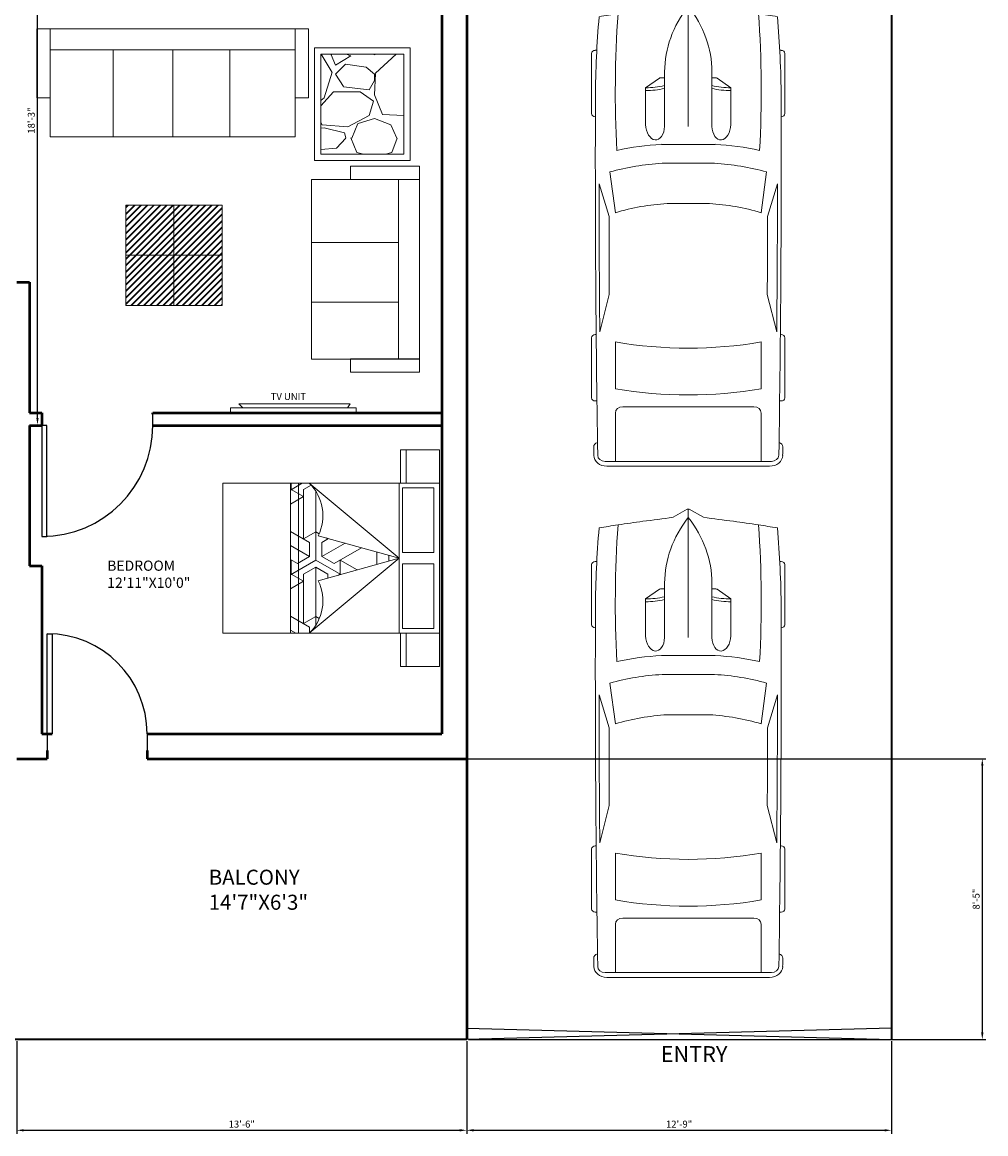
# Model space of a CAD drawing. Units: inches. Extents: x 1455 to 2044, y 1728 to 2439.
# Tile 2 of 4: x 1697 to 2044, y 1728 to 2128. Entities that reach past the tile are written whole.
import ezdxf

# ---------------------------------------------------------------- set-up
doc = ezdxf.new("R2010")
doc.units = ezdxf.units.IN
for name, color, linetype, lineweight in [('A-ANNO-DIMS', 2, 'Continuous', 18), ('A-ANNO-TEXT', 7, 'Continuous', 18), ('A-AREA-IDEN', 7, 'Continuous', 25), ('A-DOOR', 4, 'Continuous', 25), ('A-FURN', 8, 'Continuous', 18), ('A-FURN-PATT', 9, 'Continuous', 13), ('A-WALL', 7, 'Continuous', 50), ('C-PRKG-VEHI', 8, 'Continuous', 13), ('C-PROP', 7, 'Continuous', 35), ('C-SITE-GATE', 1, 'Continuous', 25)]:
    doc.layers.add(name, color=color, linetype=linetype, lineweight=lineweight)
doc.styles.get("Standard").update_dxf_attribs({"font": 'arial.ttf'})
doc.dimstyles.new('ISO-25', dxfattribs={"dimtxt": 2.5, "dimasz": 2.5, "dimexe": 1.25, "dimexo": 0.625, "dimtad": 1, "dimlunit": 3, "dimtxsty": 'Standard', "dimcen": 2.5, "dimadec": 0, "dimazin": 0, "dimtfac": 1, "dimtmove": 0, "dimatfit": 3, "dimfxl": 1, "dimarcsym": 0})

# ---------------------------------------------------------------- blocks, each defined once
blk = doc.blocks.new('*U14')
for p, q in [((0, 0), (0, -6)), ((36, 0), (36, -6))]:
    blk.add_line(p, q)
blk.add_lwpolyline([(0, 0), (0, 36), (1.75, 36), (1.75, 0)], close=True)
blk.add_arc((0, 0), 36, 0, 90)
blk = doc.blocks.new('*U13')
for p, q in [((0, 0), (0, 4)), ((40, 0), (40, 4))]:
    blk.add_line(p, q)
blk.add_lwpolyline([(0, 0), (0, -40), (1.75, -40), (1.75, 0)], close=True)
blk.add_arc((0, 0), 40, 270, 0)
blk = doc.blocks.new('*U19')
for p, q in [((21.1, 37.41), (21.1, 36.83)), ((46.55, 38.89), (22.35, 38.89)), ((47.8, 37.39), (47.8, 37.41)), ((87.99, 31.87), (74.76, 35.92)), ((135.45, 37.07), (135.45, 37.41)), ((136.7, 38.89), (160.9, 38.89)), ((162.15, 37.41), (162.15, 36.77)), ((70.03, 31.54), (86.41, 29.35)), ((134.31, 35.6), (119.29, 31.78)), ((186.47, -33.5), (186.47, 33.5)), ((188.4, -32.76), (188.4, 32.76)), ((138.42, 29.35), (157.25, 29.35)), ((186.47, 29.35), (167.01, 29.35)), ((164.52, 26.39), (164.52, -26.39)), ((32.27, 11.63), (36.13, 17.17)), ((36.13, 17.17), (50.94, 17.17)), ((29.77, 9.51), (51.68, 9.51)), ((32.12, 9.51), (32.12, 11.15)), ((58.92, -10.77), (58.92, 10.77)), ((66.55, -10.53), (66.55, 10.53)), ((186.47, -10.53), (186.47, 10.53)), ((3.27, 6.13), (0.1, 0.41)), ((82.74, 8.5), (82.74, -8.5)), ((0, 0), (51.68, 0)), ((0.1, -0.41), (3.27, -6.13)), ((29.77, -9.51), (51.68, -9.51)), ((32.12, -9.51), (32.12, -11.15)), ((32.27, -11.63), (36.13, -17.17)), ((36.13, -17.17), (50.94, -17.17)), ((86.41, -29.35), (70.03, -31.54)), ((157.25, -29.35), (138.42, -29.35)), ((167.01, -29.35), (186.47, -29.35)), ((87.99, -31.87), (74.76, -35.92)), ((134.31, -35.6), (119.29, -31.78)), ((21.1, -37.41), (21.1, -36.83)), ((46.55, -38.89), (22.35, -38.89)), ((47.8, -37.39), (47.8, -37.41)), ((135.45, -37.07), (135.45, -37.41)), ((136.7, -38.89), (160.9, -38.89)), ((162.15, -37.41), (162.15, -36.77))]:
    blk.add_line(p, q)
for centre, major_axis, ratio, start_param, end_param in [((266.03, -27.52), (0, 313.31), 0.842304, 1.367076, 1.39176), ((41.19, -490.86), (0, 528.23), 0.842304, 0.00281, 0.075598), ((22.35, 37.41), (0, -1.48), 0.842304, 3.141593, 4.712389), ((64.48, -10555.62), (0, 10593.03), 0.842304, -0.013397, 0.002797), ((46.55, 37.41), (0, 1.48), 0.842304, -1.570796, 0), ((64.48, -10555.62), (0, -10591.55), 0.842304, 3.133765, 3.140441), ((136.7, 37.41), (0, -1.48), 0.842304, 3.141593, 4.712389), ((160.9, 37.41), (0, 1.48), 0.842304, -1.570796, 0), ((180.63, 35.84), (0, 2.22), 0.842304, -0.013017, 1.249894), ((64.48, -10556.36), (0, 10595.31), 0.842304, -0.013397, -0.013017), ((183.98, 33.5), (0, -2.96), 0.842304, 1.570796, 3.128196), ((183.98, 32.76), (0, -5.25), 0.842304, 1.570796, 3.128196), ((135.29, 5.39), (0, 81.77), 0.842304, 1.245306, 1.50788), ((95.79, -3666.35), (0, -3698.24), 0.842304, 3.134049, 3.144098), ((259.18, -27.52), (0, -305.3), 0.842304, 4.528606, 4.561838), ((37.47, -593.96), (0, -623.33), 0.842304, 3.096046, 3.200911), ((134.4, 5.39), (0, -89.78), 0.842304, 4.449482, 4.652344), ((149.6, 2.8), (0, -79.58), 0.842304, 4.372215, 4.640744), ((17.08, 0), (0, 147.02), 0.842304, 4.511394, 4.913384), ((35.91, 0), (0, 147.02), 0.842304, 4.511394, 4.913384), ((167.01, 26.39), (0, 2.96), 0.842304, 0, 1.570796), ((-204.49, 52.4), (0, -250.96), 0.842304, 1.385369, 1.434372), ((13.04, 17.01), (0, 27.42), 0.842304, 4.435146, 4.718221), ((14.2, 17.01), (0, 27.42), 0.842304, 4.435146, 4.718221), ((50.79, 13.34), (6.34, -0.36), 0.603834, -1.395552, 1.581315), ((29.77, -46.66), (0, 56.17), 0.842304, 0, 0.590319), ((32.75, 11.15), (0, 0.74), 0.842304, 0.879714, 1.570796), ((0.62, 0), (0, -0.74), 0.842304, 4.131459, 5.293319), ((29.77, 46.66), (0, 56.17), 0.842304, 2.551274, 3.141593), ((-204.49, -52.4), (0, 250.96), 0.842304, -1.434372, -1.385369), ((149.6, -2.8), (0, -79.58), 0.842304, -1.499151, -1.230623), ((32.75, -11.15), (0, -0.74), 0.842304, 4.712389, 5.403472), ((13.04, -17.01), (0, -27.42), 0.842304, 1.564964, 1.848039), ((14.2, -17.01), (0, -27.42), 0.842304, 1.564964, 1.848039), ((134.4, -5.39), (0, -89.78), 0.842304, -1.510751, -1.307889), ((135.29, -5.39), (0, -81.77), 0.842304, -1.50788, -1.245306), ((259.18, 27.52), (0, 305.3), 0.842304, 1.721348, 1.754579), ((167.01, -26.39), (0, -2.96), 0.842304, 4.712389, 6.283185), ((266.03, 27.52), (0, 313.31), 0.842304, 1.749832, 1.774517), ((37.47, 593.96), (0, -623.33), 0.842304, -0.059319, 0.045547), ((64.48, 10555.62), (0, -10591.55), 0.842304, 0.001152, 0.007828), ((95.79, 3666.35), (0, -3698.24), 0.842304, -0.002505, 0.007544), ((183.98, -33.5), (0, 2.96), 0.842304, 3.15499, 4.712389), ((183.98, -32.76), (0, -5.25), 0.842304, 0.013397, 1.570796), ((41.19, 490.86), (0, -528.23), 0.842304, -0.075598, -0.00281), ((22.35, -37.41), (0, 1.48), 0.842304, 1.570796, 3.141593), ((64.48, 10555.62), (0, 10593.03), 0.842304, 3.138796, 3.15499), ((46.55, -37.41), (0, -1.48), 0.842304, 0, 1.570796), ((136.7, -37.41), (0, -1.48), 0.842304, -1.570796, 0), ((160.9, -37.41), (0, 1.48), 0.842304, 3.141593, 4.712389), ((180.63, -35.84), (0, -2.22), 0.842304, -1.249894, 0.013017), ((64.48, 10556.36), (0, 10595.31), 0.842304, 3.15461, 3.15499)]:
    blk.add_ellipse(centre, major_axis=major_axis, ratio=ratio, start_param=start_param, end_param=end_param)
at = {"extrusion": (0, 0, -1)}
blk.add_ellipse((50.79, -13.34), major_axis=(6.34, 0.36), ratio=0.603834, start_param=-1.395552, end_param=1.581315, dxfattribs=at)
blk = doc.blocks.new('*D20')
at = {"layer": 'A-ANNO-DIMS', "color": 0, "lineweight": -2, "transparency": 16777216}
for p, q in [((1702.63, 2201.77), (1703.25, 2201.77)), ((1702, 1985.27), (1702, 2199.27)), ((1702.63, 1982.77), (1703.25, 1982.77))]:
    blk.add_line(p, q, dxfattribs=at)
at = {"layer": 'A-ANNO-DIMS', "color": 0, "transparency": 16777216}
for points in [[(1701.59, 2199.27), (1702.42, 2199.27), (1702, 2201.77)], [(1701.59, 1985.27), (1702.42, 1985.27), (1702, 1982.77)]]:
    blk.add_solid(points, dxfattribs=at)
at = {"layer": 'Defpoints', "color": 0, "transparency": 16777216}
for p in [(1702, 2201.77), (1702, 2201.77), (1702, 1982.77)]:
    blk.add_point(p, dxfattribs=at)
at = {"layer": 'A-ANNO-DIMS', "color": 0, "transparency": 16777216, "insert": (1700.1, 2092.27), "char_height": 2.5, "attachment_point": 5, "rotation": 90}
blk.add_mtext('18\'-3"', dxfattribs=at)
blk = doc.blocks.new('BED-DOUBLE-WITH-NIGHTSTANDS')
h = blk.add_hatch()
h.set_pattern_fill('ESCHER', color=256, angle=-270)
h.set_pattern_definition([(150, (2210.078, -2055.985), (7e-09, -30.48), [27.94, -2.54]), (270, (2210.078, -2055.985), (26.39645, 15.24), [27.94, -2.54]), (30, (2210.078, -2055.985), (7e-09, 30.48), [27.94, -2.54]), (150, (2210.078, -2053.445), (7e-09, -30.48), [5.08, -25.4]), (30, (2210.078, -2053.445), (7e-09, 30.48), [5.08, -25.4]), (150, (2207.88, -2057.255), (7e-09, -30.48), [5.08, -25.4]), (270, (2207.88, -2057.255), (26.39645, 15.24), [5.08, -25.4]), (30, (2212.278, -2057.255), (7e-09, 30.48), [5.08, -25.4]), (270, (2212.278, -2057.255), (26.39645, 15.24), [5.08, -25.4]), (150, (2210.078, -2066.145), (7e-09, -30.48), [5.08, -25.4]), (30, (2210.078, -2066.145), (7e-09, 30.48), [5.08, -25.4]), (150, (2218.877, -2050.905), (7e-09, -30.48), [5.08, -25.4]), (270, (2218.877, -2050.905), (26.39645, 15.24), [5.08, -25.4]), (30, (2201.28, -2050.905), (7e-09, 30.48), [5.08, -25.4]), (270, (2201.28, -2050.905), (26.39645, 15.24), [5.08, -25.4]), (90, (2205.68, -2050.905), (-26.39645, -15.24), [17.78, -12.7]), (90, (2214.478, -2050.905), (-26.39645, -15.24), [17.78, -12.7]), (210, (2203.48, -2054.715), (-7e-09, -30.48), [17.78, -12.7]), (210, (2207.88, -2062.335), (-7e-09, -30.48), [17.78, -12.7]), (330, (2212.278, -2062.335), (26.39645, 15.24), [17.78, -12.7]), (330, (2216.678, -2054.715), (26.39645, 15.24), [17.78, -12.7])])
h.paths.add_polyline_path([(-31.09, 54, 0.326433), (-34.36, 35.12), (-63.46, 27), (-34.36, 18.88, 0.326433), (-31.09, 0), (-27.21, 0), (-27.21, 54)])
h.paths.add_polyline_path([(-27.21, 54), (-27.21, 0), (-24.3, 0), (-24.3, 54)])
for p, q in [((-78, 54), (-78, 66)), ((-78, 66), (-66, 66)), ((-66, 66), (-66, 54)), ((-66, 66), (-64, 66)), ((-64, 66), (-64, 54)), ((-63.46, 0), (-63.46, 54)), ((-63.46, 27), (-31.09, 54)), ((-63.46, 27), (-34.36, 35.12)), ((-76.01, 28.95), (-64.69, 28.95)), ((-76.01, 24.95), (-64.69, 24.95)), ((-63.46, 27), (-31.09, 0)), ((-63.46, 27), (-34.36, 18.88)), ((-78, 0), (-78, -12)), ((-66, -12), (-66, 0)), ((-64, -12), (-64, 0)), ((-78, -12), (-66, -12)), ((-66, -12), (-64, -12))]:
    blk.add_line(p, q)
for points in [[(0, 0), (0, 54), (-78, 54), (-78, 0)], [(-27.21, 0), (-27.21, 54), (-24.3, 54), (-24.3, 0)]]:
    blk.add_lwpolyline(points, close=True)
for points in [[(-76.01, 28.95), (-76.01, 52.28), (-64.69, 52.28), (-64.69, 28.95)], [(-64.69, 24.95), (-64.69, 1.63), (-76.01, 1.63), (-76.01, 24.95)]]:
    blk.add_lwpolyline(points)
for centre, start, end in [((-19.81, 42.32), 134.0109, 206.3245), ((-19.81, 11.68), 153.6755, 225.9891)]:
    blk.add_arc(centre, 16.24, start, end)
blk = doc.blocks.new('*D27')
at = {"layer": 'A-ANNO-DIMS', "color": 0, "lineweight": -2, "transparency": 16777216}
for p, q in [((1856.58, 1760.95), (1856.58, 1727.63)), ((2009.58, 1760.95), (2009.58, 1727.63)), ((1859.08, 1728.88), (2007.08, 1728.88))]:
    blk.add_line(p, q, dxfattribs=at)
at = {"layer": 'A-ANNO-DIMS', "color": 0, "transparency": 16777216}
for points in [[(1859.08, 1729.3), (1859.08, 1728.46), (1856.58, 1728.88)], [(2007.08, 1729.3), (2007.08, 1728.46), (2009.58, 1728.88)]]:
    blk.add_solid(points, dxfattribs=at)
at = {"layer": 'Defpoints', "color": 0, "transparency": 16777216}
for p in [(1856.58, 1761.58), (2009.58, 1761.58), (2009.58, 1728.88)]:
    blk.add_point(p, dxfattribs=at)
at = {"layer": 'A-ANNO-DIMS', "color": 0, "transparency": 16777216, "insert": (1933.08, 1730.78), "char_height": 2.5, "attachment_point": 5}
blk.add_mtext('12\'-9"', dxfattribs=at)
blk = doc.blocks.new('*D28')
at = {"layer": 'A-ANNO-DIMS', "color": 0, "lineweight": -2, "transparency": 16777216}
for p, q in [((1694.58, 1760.95), (1694.58, 1727.63)), ((1856.58, 1760.95), (1856.58, 1727.63)), ((1697.08, 1728.88), (1854.08, 1728.88))]:
    blk.add_line(p, q, dxfattribs=at)
at = {"layer": 'A-ANNO-DIMS', "color": 0, "transparency": 16777216}
for points in [[(1697.08, 1729.3), (1697.08, 1728.46), (1694.58, 1728.88)], [(1854.08, 1729.3), (1854.08, 1728.46), (1856.58, 1728.88)]]:
    blk.add_solid(points, dxfattribs=at)
at = {"layer": 'Defpoints', "color": 0, "transparency": 16777216}
for p in [(1694.58, 1761.58), (1856.58, 1761.58), (1856.58, 1728.88)]:
    blk.add_point(p, dxfattribs=at)
at = {"layer": 'A-ANNO-DIMS', "color": 0, "transparency": 16777216, "insert": (1775.58, 1730.78), "char_height": 2.5, "attachment_point": 5}
blk.add_mtext('13\'-6"', dxfattribs=at)
blk = doc.blocks.new('*D31')
at = {"layer": 'A-ANNO-DIMS', "color": 0, "lineweight": -2, "transparency": 16777216}
for p, q in [((1857.2, 1862.58), (2043.53, 1862.58)), ((2042.28, 1860.08), (2042.28, 1764.08)), ((1857.2, 1761.58), (2043.53, 1761.58))]:
    blk.add_line(p, q, dxfattribs=at)
at = {"layer": 'A-ANNO-DIMS', "color": 0, "transparency": 16777216}
for points in [[(2041.86, 1860.08), (2042.7, 1860.08), (2042.28, 1862.58)], [(2041.86, 1764.08), (2042.7, 1764.08), (2042.28, 1761.58)]]:
    blk.add_solid(points, dxfattribs=at)
at = {"layer": 'Defpoints', "color": 0, "transparency": 16777216}
for p in [(1856.58, 1862.58), (1856.58, 1761.58), (2042.28, 1761.58)]:
    blk.add_point(p, dxfattribs=at)
at = {"layer": 'A-ANNO-DIMS', "color": 0, "transparency": 16777216, "insert": (2040.38, 1812.08), "char_height": 2.5, "attachment_point": 5, "rotation": 90}
blk.add_mtext('8\'-5"', dxfattribs=at)

msp = doc.modelspace()

# ---------------------------------------------------------------- hatches: boundary and pattern name
at = {"layer": 'A-FURN-PATT'}
h = msp.add_hatch(dxfattribs=at)
h.set_pattern_fill('GRAVEL', color=256, scale=1.455478)
h.set_pattern_definition([(228.01279, (777.6254, 1161.526), (-295.7530417, -332.722172), [4.9737, -492.3951]), (184.96974, (774.2982, 1157.829), (443.6295623, 36.9691323), [8.535, -844.96366]), (132.51045, (765.7953, 1157.0896), (369.6913022, -406.660432), [6.0181, -595.7957]), (267.27369, (751.3773, 1147.8473), (36.9691303, 739.382604), [7.7723, -769.45914]), (292.83365, (751.0076, 1140.0838), (-184.845651, 443.6295624), [7.6214, -754.5168]), (357.27369, (753.9652, 1133.0597), (-739.382604, 36.9691303), [7.7723, -769.45914]), (37.69424, (761.7287, 1132.69), (-480.5986926, -369.6913021), [10.2785, -1017.5697]), (72.25533, (769.8619, 1138.9747), (258.7839115, 813.3208645), [9.70395, -960.6917]), (121.42957, (772.8194, 1148.217), (-295.7530417, 480.5986926), [7.79864, -772.066]), (175.23636, (768.7528, 1154.8714), (406.660432, -36.96913), [8.90335, -436.2639]), (222.39744, (759.8802, 1155.6108), (-443.6295624, -406.6604323), [11.51396, -1139.88306]), (138.81407, (787.9768, 1147.4776), (-258.783911, 221.814781), [3.92986, -389.0574]), (171.46923, (785.0192, 1150.0655), (480.5986927, -73.9382603), [7.4765, -740.17786]), (225, (777.625, 1151.175), (-5e-15, -36.96913), [5.2282, -47.054]), (203.1986, (775.0376, 1155.611), (184.845651, 73.93826), [2.8155, -278.733]), (291.8014, (772.45, 1154.502), (-36.96913, 110.90739), [3.9817, -195.1032]), (30.96376, (773.9285, 1150.805), (110.90739, 73.93826), [6.467, -209.09825]), (161.56505, (779.474, 1154.132), (73.93826, -36.96913), [4.6763, -112.2304]), (16.38954, (751.0076, 1154.5017), (369.691302, 110.9073906), [6.5509, -648.5437]), (70.34618, (757.2924, 1156.3502), (-147.876521, -406.6604322), [5.4959, -544.08976]), (293.1986, (779.474, 1161.526), (-73.93826, 184.845651), [5.63095, -275.91755]), (343.61046, (781.692, 1156.3502), (-369.691302, 110.9073906), [6.5509, -648.5437]), (339.44395, (751.0076, 1131.581), (-184.845651, 73.93826), [6.3173, -309.5471]), (294.77514, (756.9227, 1129.3627), (-184.8456512, 406.660432), [5.2932, -524.0242]), (66.8014, (779.8435, 1124.5568), (73.93826, 184.845651), [5.63095, -275.91755]), (17.35402, (782.0617, 1129.7324), (-480.5986926, -147.876521), [6.1972, -613.5184]), (69.44395, (761.7287, 1124.5568), (-73.93826, -184.845651), [3.15864, -312.70574]), (101.30993, (777.6254, 1124.557), (-36.96913, 147.87652), [1.88506, -186.6213]), (165.96376, (777.256, 1126.405), (110.90739, -36.96913), [7.6214, -144.8063]), (186.009, (769.8619, 1128.2537), (369.691302, 36.9691302), [7.06295, -699.2313]), (303.6901, (773.928, 1147.478), (-36.96913, 73.93826), [5.3318, -127.9623]), (353.15723, (776.886, 1143.0413), (628.4752135, -73.9382604), [9.3086, -921.5503]), (60.9454, (786.1283, 1141.9322), (-147.876521, -258.783911), [3.8062, -376.8143]), (90, (787.977, 1145.26), (-36.9691, 36.9691), [2.21815, -34.751]), (120.25644, (769.1225, 1129.3627), (147.876521, -258.7839114), [5.1359, -508.4557]), (48.01279, (766.5347, 1133.799), (295.7530417, 332.722172), [9.94736, -487.4214]), (0, (773.19, 1141.193), (36.9691, 36.9691), [9.612, -27.3572]), (325.30485, (782.801, 1141.1929), (369.691302, -258.7839112), [5.84534, -578.68794]), (254.0546, (787.607, 1137.8656), (-36.96913, -147.87652), [5.3828, -263.75655]), (207.64598, (786.1283, 1132.69), (-702.4134739, -369.691302), [8.7641, -867.64605]), (175.42608, (778.3648, 1128.6234), (-480.5986926, 36.9691302), [9.2718, -917.90925])])
h.paths.add_polyline_path([(1833.918, 2116.122), (1804.032, 2116.122), (1804.032, 2080.131), (1833.918, 2080.131)])
h = msp.add_hatch(dxfattribs=at)
h.set_pattern_fill('JIS_RC_10', color=256, scale=0.163741)
h.set_pattern_definition([(45, (751.0076, 1124.5568), (-1.1578253, 1.1578253), []), (45, (751.1263, 1124.5568), (-1.1578253, 1.1578253), []), (45, (751.245, 1124.5568), (-1.1578253, 1.1578253), [])])
h.paths.add_polyline_path([(1768.479, 2061.828), (1751.143, 2061.828), (1751.143, 2043.796), (1768.479, 2043.796)])
h.paths.add_polyline_path([(1751.143, 2043.796), (1733.808, 2043.796), (1733.808, 2025.764), (1751.143, 2025.764)])
h.paths.add_polyline_path([(1768.479, 2043.796), (1751.143, 2043.796), (1751.143, 2025.764), (1768.479, 2025.764)])
h.paths.add_polyline_path([(1751.143, 2061.828), (1733.808, 2061.828), (1733.808, 2043.796), (1751.143, 2043.796)])

# ---------------------------------------------------------------- linework, layer by layer
at = {"layer": 'A-FURN'}
for p, q in [((1729.283, 2117.78), (1729.283, 2086.419)), ((1750.722, 2117.78), (1750.722, 2086.419)), ((1771.306, 2117.78), (1771.306, 2086.419)), ((1751.143, 2061.828), (1751.143, 2025.764)), ((1832.05, 2048.411), (1800.689, 2048.411)), ((1733.808, 2043.796), (1768.479, 2043.796)), ((1832.05, 2026.972), (1800.689, 2026.972)), ((1832.05, 2006.387), (1800.689, 2006.387)), ((1832.05, 2006.387), (1839.542, 2006.387)), ((1814.596, 1990.363), (1774.487, 1990.363)), ((1774.487, 1990.363), (1776.002, 1988.943)), ((1813.613, 1988.943), (1814.596, 1990.363))]:
    msp.add_line(p, q, dxfattribs=at)
for points in [[(1706.615, 2125.272), (1701.774, 2125.272), (1701.774, 2100.457), (1706.615, 2100.457)], [(1706.615, 2117.78), (1794.858, 2117.78), (1794.858, 2125.272), (1706.615, 2125.272)], [(1799.67, 2125.272), (1794.828, 2125.272), (1794.828, 2100.457), (1799.67, 2100.457)], [(1706.615, 2117.78), (1794.828, 2117.78), (1794.828, 2086.419), (1706.615, 2086.419)], [(1801.758, 2118.396), (1836.192, 2118.396), (1836.192, 2077.857), (1801.758, 2077.857)], [(1804.032, 2116.122), (1833.918, 2116.122), (1833.918, 2080.131), (1804.032, 2080.131)], [(1839.542, 2071.078), (1839.542, 2075.92), (1814.727, 2075.92), (1814.727, 2071.078)], [(1733.808, 2061.828), (1768.479, 2061.828), (1768.479, 2025.764), (1733.808, 2025.764)], [(1839.542, 2001.714), (1839.542, 2006.555), (1814.727, 2006.555), (1814.727, 2001.714)], [(1771.53, 1987.079), (1816.742, 1987.079), (1816.742, 1988.943), (1771.53, 1988.943)]]:
    msp.add_lwpolyline(points, close=True, dxfattribs=at)
for points in [[(1800.689, 2006.387), (1800.689, 2071.078), (1832.05, 2071.078), (1832.05, 2006.387)], [(1839.542, 2006.387), (1839.542, 2071.078), (1832.05, 2071.078), (1832.05, 2006.387)]]:
    msp.add_lwpolyline(points, dxfattribs=at)
at = {"layer": 'A-WALL'}
for p, q in [((1856.58, 2340.579), (1856.58, 1770.579)), ((1847.58, 2244.579), (1847.58, 1871.579)), ((1694.58, 2034.079), (1699.08, 2034.079)), ((1699.08, 2034.079), (1699.08, 1987.079)), ((1703.578, 1986.569), (1703.578, 1987.079)), ((1703.58, 1987.079), (1703.58, 1982.579)), ((1743.578, 1986.569), (1743.578, 1987.079)), ((1699.08, 1982.579), (1699.08, 1932.079)), ((1699.08, 1932.079), (1703.58, 1932.079)), ((1703.58, 1932.079), (1703.58, 1923.079)), ((1703.58, 1923.079), (1703.58, 1871.579)), ((1705.504, 1865.579), (1705.504, 1862.579)), ((1741.504, 1865.579), (1741.504, 1862.579)), ((1847.58, 1862.579), (1856.58, 1862.579)), ((1856.58, 1770.579), (1856.58, 1761.579))]:
    msp.add_line(p, q, dxfattribs=at)
for points in [[(1699.08, 1987.079), (1703.58, 1987.079)], [(1743.578, 1987.079), (1793.58, 1987.079), (1847.58, 1987.079)], [(1699.08, 1982.579), (1703.58, 1982.579)], [(1743.578, 1982.579), (1793.58, 1982.579), (1847.58, 1982.579)], [(1703.58, 1871.579), (1707.254, 1871.579)], [(1741.504, 1871.579), (1793.58, 1871.579), (1847.58, 1871.579)], [(1694.58, 1862.579), (1705.504, 1862.579)], [(1741.504, 1862.579), (1793.58, 1862.579), (1847.58, 1862.579)]]:
    msp.add_lwpolyline(points, dxfattribs=at)
at = {"layer": 'C-PROP'}
for p, q in [((2009.58, 2349.579), (2009.58, 1761.579)), ((1856.58, 1761.579), (1505.58, 1761.579))]:
    msp.add_line(p, q, dxfattribs=at)
at = {"layer": 'C-SITE-GATE'}
for p, q in [((1856.58, 1765.579), (2009.58, 1761.579)), ((2009.528, 1765.579), (1856.58, 1761.579)), ((2009.58, 1761.579), (2009.528, 1765.579))]:
    msp.add_line(p, q, dxfattribs=at)

# ---------------------------------------------------------------- block references
at = {"layer": 'A-DOOR'}
for name, p in [('*U13', (1703.578, 1982.569)), ('*U14', (1705.504, 1871.579))]:
    msp.add_blockref(name, p, dxfattribs=at)
at = {"layer": 'A-FURN', "rotation": 180}
msp.add_blockref('BED-DOUBLE-WITH-NIGHTSTANDS', (1768.779, 1961.748), dxfattribs=at)
at = {"layer": 'C-PRKG-VEHI', "xscale": 0.8946429665525277, "yscale": 0.8946429665525277, "zscale": 0.8946429665525277, "rotation": 270}
for p in [(1936.381, 2136.429), (1936.381, 1952.454)]:
    msp.add_blockref('*U19', p, dxfattribs=at)

# ---------------------------------------------------------------- texts
at = {"layer": 'A-ANNO-TEXT', "attachment_point": 1}
for s, width, gutter_width, insert, char_height in [('TV UNIT', 17.72271, 12.5, (1786.017, 1994.214), 2.5), ('ENTRY', 92.73423, 28.611, (1926.468, 1759.166), 5.7222)]:
    msp.add_mtext_dynamic_manual_height_columns(s, width=width, gutter_width=gutter_width, heights=[0], dxfattribs=dict(at, insert=insert, char_height=char_height))
at = {"layer": 'A-AREA-IDEN', "attachment_point": 1}
for s, width, gutter_width, insert, char_height in [('BEDROOM\\P12\'11"X10\'0"', 54.1231, 18.405, (1727.134, 1933.921), 3.68098), ('BALCONY\\P14\'7"X6\'3"', 143.92766, 27.03, (1763.679, 1822.669), 5.4059)]:
    msp.add_mtext_dynamic_manual_height_columns(s, width=width, gutter_width=gutter_width, heights=[0], dxfattribs=dict(at, insert=insert, char_height=char_height))

# ---------------------------------------------------------------- dimensions: what is measured, and where the dimension line sits
at = {"layer": 'A-ANNO-DIMS'}
for base, p1, p2, override, picture, middle in [((1702.002, 2201.769), (1702.002, 1982.769), (1702.002, 2201.769), {"dimclrd": 0, "dimclre": 0, "dimclrt": 0}, '*D20', (1700.099, 2092.269)), ((2042.28, 1761.579), (1856.58, 1862.579), (1856.58, 1761.579), {"dimdec": 1, "dimlfac": 1, "dimrnd": 0, "dimzin": 1, "dimdsep": 46, "dimlunit": 4, "dimfrac": 2}, '*D31', (2040.378, 1812.079))]:
    dim = msp.add_linear_dim(base=base, p1=p1, p2=p2, angle=90, dimstyle='ISO-25', override=override, dxfattribs=at)
    dim.commit()
    dim.dimension.update_dxf_attribs({"geometry": picture, "text_midpoint": middle})
for base, p1, p2, picture, middle in [((1856.58, 1728.879), (1694.58, 1761.579), (1856.58, 1761.579), '*D28', (1775.58, 1730.781)), ((2009.58, 1728.879), (1856.58, 1761.579), (2009.58, 1761.579), '*D27', (1933.08, 1730.78))]:
    dim = msp.add_linear_dim(base=base, p1=p1, p2=p2, dimstyle='ISO-25', override={"dimdec": 1, "dimlfac": 1, "dimrnd": 0, "dimzin": 1, "dimdsep": 46, "dimlunit": 4, "dimfrac": 2}, dxfattribs=at)
    dim.commit()
    dim.dimension.update_dxf_attribs({"geometry": picture, "text_midpoint": middle})

doc.saveas('drawing.dxf')
